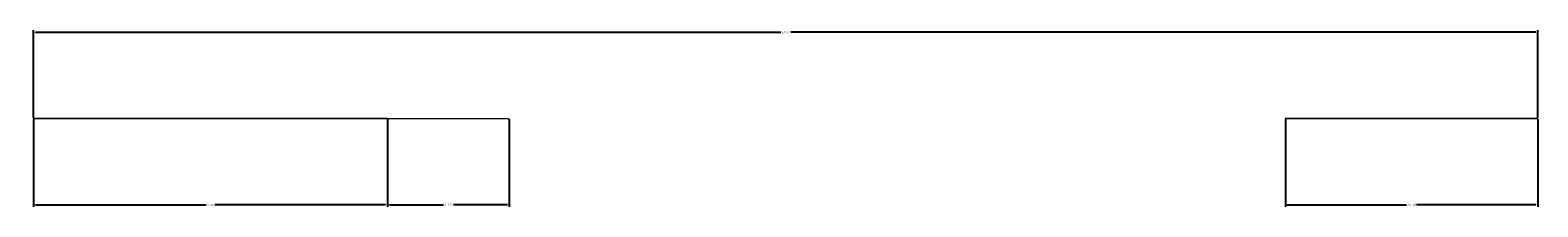
# Model space of a CAD drawing. Units: millimetres. Extents: x 498 to 637, y -8 to 8.
import ezdxf

# ---------------------------------------------------------------- set-up
doc = ezdxf.new("R2010")
doc.units = ezdxf.units.MM
doc.layers.add('M-CONS', color=8, linetype='Continuous', lineweight=13)
doc.layers.add('M-DIMS', color=2, linetype='Continuous', lineweight=18)
doc.styles.get("Standard").update_dxf_attribs({"font": 'arial.ttf'})
doc.dimstyles.get("Standard").update_dxf_attribs({"dimtxt": 0.18, "dimasz": 0.18, "dimexe": 0.18, "dimexo": 0.0625, "dimgap": 0.09, "dimtad": 0, "dimtih": 1, "dimtoh": 1, "dimdec": 4, "dimzin": 0, "dimdsep": 46, "dimtxsty": 'Standard', "dimcen": 0.09, "dimadec": 0, "dimazin": 0, "dimtfac": 1, "dimtdec": 4, "dimtofl": 0, "dimtmove": 0, "dimatfit": 3, "dimfxl": 1, "dimtolj": 1, "dimtzin": 0, "dimarcsym": 0})

# ---------------------------------------------------------------- blocks, each defined once
blk = doc.blocks.new('*D1')
at = {"layer": 'Defpoints', "color": 0, "transparency": 16777216}
for p in [(636.68, 7.9), (498.71, 0), (636.68, 0)]:
    blk.add_point(p, dxfattribs=at)
at = {"layer": 'M-DIMS', "color": 0, "lineweight": -2, "transparency": 16777216}
for p, q in [((498.71, 0.06), (498.71, 8.08)), ((498.89, 7.9), (567.24, 7.9)), ((636.5, 7.9), (568.15, 7.9)), ((636.68, 0.06), (636.68, 8.08))]:
    blk.add_line(p, q, dxfattribs=at)
at = {"layer": 'M-DIMS', "color": 0, "transparency": 16777216}
for points in [[(498.89, 7.93), (498.89, 7.87), (498.71, 7.9)], [(636.5, 7.93), (636.5, 7.87), (636.68, 7.9)]]:
    blk.add_solid(points, dxfattribs=at)
at = {"layer": 'M-DIMS', "color": 0, "transparency": 16777216, "insert": (567.69, 7.9), "char_height": 0.18, "attachment_point": 5}
blk.add_mtext('\\A1;137.97', dxfattribs=at)
blk = doc.blocks.new('*D2')
at = {"layer": 'Defpoints', "color": 0, "transparency": 16777216}
for p in [(498.71, 0), (531.17, 0), (531.17, -7.9)]:
    blk.add_point(p, dxfattribs=at)
at = {"layer": 'M-DIMS', "color": 0, "lineweight": -2, "transparency": 16777216}
for p, q in [((498.71, -0.06), (498.71, -8.08)), ((531.17, -0.06), (531.17, -8.08)), ((498.89, -7.9), (514.55, -7.9)), ((530.99, -7.9), (515.33, -7.9))]:
    blk.add_line(p, q, dxfattribs=at)
at = {"layer": 'M-DIMS', "color": 0, "transparency": 16777216}
for points in [[(498.89, -7.87), (498.89, -7.93), (498.71, -7.9)], [(530.99, -7.87), (530.99, -7.93), (531.17, -7.9)]]:
    blk.add_solid(points, dxfattribs=at)
at = {"layer": 'M-DIMS', "color": 0, "transparency": 16777216, "insert": (514.94, -7.9), "char_height": 0.18, "attachment_point": 5}
blk.add_mtext('\\A1;32.46', dxfattribs=at)
blk = doc.blocks.new('*D3')
at = {"layer": 'Defpoints', "color": 0, "transparency": 16777216}
for p in [(531.17, 0), (542.34, 0), (542.34, -7.9)]:
    blk.add_point(p, dxfattribs=at)
at = {"layer": 'M-DIMS', "color": 0, "lineweight": -2, "transparency": 16777216}
for p, q in [((531.17, -0.06), (531.17, -8.08)), ((542.34, -0.06), (542.34, -8.08)), ((531.35, -7.9), (536.3, -7.9)), ((542.16, -7.9), (537.21, -7.9))]:
    blk.add_line(p, q, dxfattribs=at)
at = {"layer": 'M-DIMS', "color": 0, "transparency": 16777216}
for points in [[(531.35, -7.87), (531.35, -7.93), (531.17, -7.9)], [(542.16, -7.87), (542.16, -7.93), (542.34, -7.9)]]:
    blk.add_solid(points, dxfattribs=at)
at = {"layer": 'M-DIMS', "color": 0, "transparency": 16777216, "insert": (536.76, -7.9), "char_height": 0.18, "attachment_point": 5}
blk.add_mtext('\\A1;11.172', dxfattribs=at)
blk = doc.blocks.new('*D4')
at = {"layer": 'Defpoints', "color": 0, "transparency": 16777216}
for p in [(613.52, 0), (636.68, 0), (636.68, -7.9)]:
    blk.add_point(p, dxfattribs=at)
at = {"layer": 'M-DIMS', "color": 0, "lineweight": -2, "transparency": 16777216}
for p, q in [((613.52, -0.06), (613.52, -8.08)), ((636.68, -0.06), (636.68, -8.08)), ((613.7, -7.9), (624.63, -7.9)), ((636.5, -7.9), (625.56, -7.9))]:
    blk.add_line(p, q, dxfattribs=at)
at = {"layer": 'M-DIMS', "color": 0, "transparency": 16777216}
for points in [[(613.7, -7.87), (613.7, -7.93), (613.52, -7.9)], [(636.5, -7.87), (636.5, -7.93), (636.68, -7.9)]]:
    blk.add_solid(points, dxfattribs=at)
at = {"layer": 'M-DIMS', "color": 0, "transparency": 16777216, "insert": (625.1, -7.9), "char_height": 0.18, "attachment_point": 5}
blk.add_mtext('\\A1;23.164', dxfattribs=at)

msp = doc.modelspace()

# ---------------------------------------------------------------- linework, layer by layer
at = {"layer": 'M-CONS', "extrusion": (0, -1, 0)}
msp.add_lwpolyline([(523.6711, 136.9572, -0.37824245), (513.7483, 145.7168), (498.7483, 265.7168, -0.45112349), (508.6711, 276.9572), (522.3433, 276.9572, -0.41421356), (532.3433, 266.9572), (532.3433, 206.9572, 0.41421356), (542.3433, 196.9572), (542.3433, 136.9572)], format="xyb", dxfattribs=at)
for centre in [(515.5072, 256.9572), (523.6711, 156.9572), (621.0155, 156.9572), (629.1794, 256.9572)]:
    msp.add_circle(centre, 7.5, dxfattribs=at)

# ---------------------------------------------------------------- dimensions: what is measured, and where the dimension line sits
at = {"layer": 'M-DIMS'}
for base, p1, p2, override, picture, middle in [((636.6794, 7.9), (498.7104, 0), (636.6794, 0), {"dimdec": 2, "dimlfac": 1, "dimrnd": 0, "dimzin": 0, "dimdsep": 46, "dimlunit": 2}, '*D1', (567.6949, 7.9)), ((531.1711, -7.9), (498.7104, 0), (531.1711, 0), {"dimdec": 2, "dimlfac": 1, "dimrnd": 0, "dimzin": 0, "dimdsep": 46, "dimlunit": 2}, '*D2', (514.9408, -7.9)), ((542.3433, -7.9), (531.1711, 0), (542.3433, 0), {"dimdec": 3, "dimlfac": 1, "dimrnd": 0, "dimzin": 0, "dimdsep": 46, "dimlunit": 2}, '*D3', (536.7572, -7.9)), ((636.6794, -7.9), (613.5155, 0), (636.6794, 0), {"dimdec": 3, "dimlfac": 1, "dimrnd": 0, "dimzin": 0, "dimdsep": 46, "dimlunit": 2}, '*D4', (625.0974, -7.9))]:
    dim = msp.add_linear_dim(base=base, p1=p1, p2=p2, dimstyle='Standard', override=override, dxfattribs=at)
    dim.commit()
    dim.dimension.update_dxf_attribs({"geometry": picture, "text_midpoint": middle})

doc.saveas('drawing.dxf')
